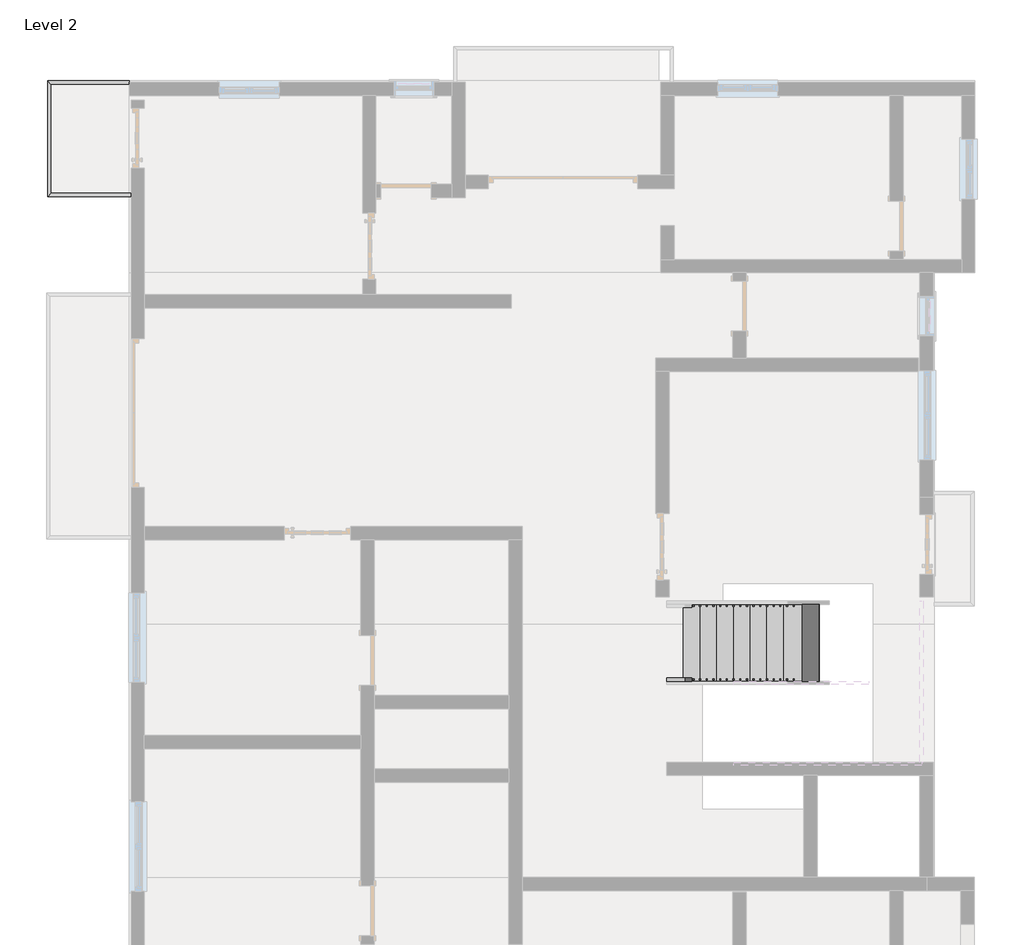
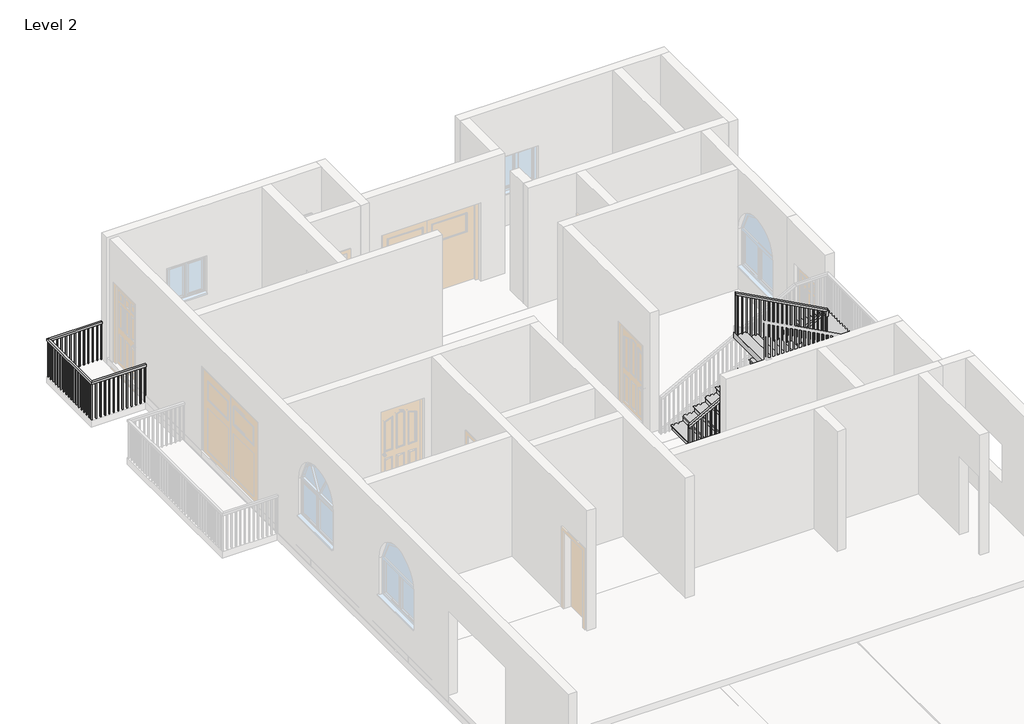
# One storey, part 5 of 7: 2 railings, 1 stair flight.
"""IFC4 building model written with IfcOpenShell, lengths in millimetres."""

from ifc_helpers import new_model, si_unit, frame, origin, place, context, project, spatial, polyline, outline, extrude, faceted_brep, transform, mapped, element, save
from components import stair_flight_e3e94c6b

model = new_model("IFC4")

# Units and contexts
model_context = context("Model", 3, world=origin())
ifc_project = project(units=[si_unit("LENGTHUNIT", "METRE", prefix="MILLI")], contexts=[model_context])

# Site, building, storey
site = spatial("IfcSite", under=ifc_project)
building = spatial("IfcBuilding", under=site)
storey = spatial("IfcBuildingStorey", under=building, Name="Level 2", Elevation=3048.0)

# Railings
placement = place(None, origin())
element("IfcRailing", 1, ObjectType="Handrail - Rectangular", at=placement, inside=storey, context=model_context, shape_type="SolidModel", body=[
    faceted_brep([(-6354.2109037, 9376.4527313, 3962.4), (-6354.2109037, 9376.4527313, 3911.6), (-6354.2109037, 9427.2527313, 3911.6), (-6354.2109037, 9427.2527313, 3962.4), (-7548.0109037, 9376.4527313, 3962.4), (-7548.0109037, 9376.4527313, 3911.6), (-7598.8109037, 9427.2527313, 3911.6), (-7598.8109037, 9427.2527313, 3962.4), (-7548.0109037, 7717.9584215, 3962.4), (-7548.0109037, 7717.9584215, 3911.6), (-7598.8109037, 7667.1584215, 3911.6), (-7598.8109037, 7667.1584215, 3962.4), (-6330.8013636, 7717.9584215, 3962.4), (-6330.8013636, 7667.1584215, 3962.4), (-6330.8013636, 7667.1584215, 3911.6), (-6330.8013636, 7717.9584215, 3911.6)], [[[0, 1, 2, 3]], [[1, 0, 4, 5]], [[2, 1, 5, 6]], [[3, 2, 6, 7]], [[0, 3, 7, 4]], [[5, 4, 8, 9]], [[6, 5, 9, 10]], [[7, 6, 10, 11]], [[4, 7, 11, 8]], [[12, 13, 14, 15]], [[9, 8, 12, 15]], [[10, 9, 15, 14]], [[11, 10, 14, 13]], [[8, 11, 13, 12]]]),
    extrude(outline(polyline([(-6363.7359037, 7683.0334215), (-6363.7359037, 7702.0834215), (-6344.6859037, 7702.0834215), (-6344.6859037, 7683.0334215), (-6363.7359037, 7683.0334215)])), frame((0.0, 0.0, 3048.0), z_axis=(0.0, 0.0, 1.0), x_axis=(1.0, 0.0, 0.0)), (0.0, 0.0, 1.0), 863.6),
    extrude(outline(polyline([(-6465.3359037, 7683.0334215), (-6465.3359037, 7702.0834215), (-6446.2859037, 7702.0834215), (-6446.2859037, 7683.0334215), (-6465.3359037, 7683.0334215)])), frame((0.0, 0.0, 3048.0), z_axis=(0.0, 0.0, 1.0), x_axis=(1.0, 0.0, 0.0)), (0.0, 0.0, 1.0), 863.6),
    extrude(outline(polyline([(-6566.9359037, 7683.0334215), (-6566.9359037, 7702.0834215), (-6547.8859037, 7702.0834215), (-6547.8859037, 7683.0334215), (-6566.9359037, 7683.0334215)])), frame((0.0, 0.0, 3048.0), z_axis=(0.0, 0.0, 1.0), x_axis=(1.0, 0.0, 0.0)), (0.0, 0.0, 1.0), 863.6),
    extrude(outline(polyline([(-6668.5359037, 7683.0334215), (-6668.5359037, 7702.0834215), (-6649.4859037, 7702.0834215), (-6649.4859037, 7683.0334215), (-6668.5359037, 7683.0334215)])), frame((0.0, 0.0, 3048.0), z_axis=(0.0, 0.0, 1.0), x_axis=(1.0, 0.0, 0.0)), (0.0, 0.0, 1.0), 863.6),
    extrude(outline(polyline([(-6770.1359037, 7683.0334215), (-6770.1359037, 7702.0834215), (-6751.0859037, 7702.0834215), (-6751.0859037, 7683.0334215), (-6770.1359037, 7683.0334215)])), frame((0.0, 0.0, 3048.0), z_axis=(0.0, 0.0, 1.0), x_axis=(1.0, 0.0, 0.0)), (0.0, 0.0, 1.0), 863.6),
    extrude(outline(polyline([(-6871.7359037, 7683.0334215), (-6871.7359037, 7702.0834215), (-6852.6859037, 7702.0834215), (-6852.6859037, 7683.0334215), (-6871.7359037, 7683.0334215)])), frame((0.0, 0.0, 3048.0), z_axis=(0.0, 0.0, 1.0), x_axis=(1.0, 0.0, 0.0)), (0.0, 0.0, 1.0), 863.6),
    extrude(outline(polyline([(-6973.3359037, 7683.0334215), (-6973.3359037, 7702.0834215), (-6954.2859037, 7702.0834215), (-6954.2859037, 7683.0334215), (-6973.3359037, 7683.0334215)])), frame((0.0, 0.0, 3048.0), z_axis=(0.0, 0.0, 1.0), x_axis=(1.0, 0.0, 0.0)), (0.0, 0.0, 1.0), 863.6),
    extrude(outline(polyline([(-7074.9359037, 7683.0334215), (-7074.9359037, 7702.0834215), (-7055.8859037, 7702.0834215), (-7055.8859037, 7683.0334215), (-7074.9359037, 7683.0334215)])), frame((0.0, 0.0, 3048.0), z_axis=(0.0, 0.0, 1.0), x_axis=(1.0, 0.0, 0.0)), (0.0, 0.0, 1.0), 863.6),
    extrude(outline(polyline([(-7176.5359037, 7683.0334215), (-7176.5359037, 7702.0834215), (-7157.4859037, 7702.0834215), (-7157.4859037, 7683.0334215), (-7176.5359037, 7683.0334215)])), frame((0.0, 0.0, 3048.0), z_axis=(0.0, 0.0, 1.0), x_axis=(1.0, 0.0, 0.0)), (0.0, 0.0, 1.0), 863.6),
    extrude(outline(polyline([(-7278.1359037, 7683.0334215), (-7278.1359037, 7702.0834215), (-7259.0859037, 7702.0834215), (-7259.0859037, 7683.0334215), (-7278.1359037, 7683.0334215)])), frame((0.0, 0.0, 3048.0), z_axis=(0.0, 0.0, 1.0), x_axis=(1.0, 0.0, 0.0)), (0.0, 0.0, 1.0), 863.6),
    extrude(outline(polyline([(-7379.7359037, 7683.0334215), (-7379.7359037, 7702.0834215), (-7360.6859037, 7702.0834215), (-7360.6859037, 7683.0334215), (-7379.7359037, 7683.0334215)])), frame((0.0, 0.0, 3048.0), z_axis=(0.0, 0.0, 1.0), x_axis=(1.0, 0.0, 0.0)), (0.0, 0.0, 1.0), 863.6),
    extrude(outline(polyline([(-7481.3359037, 7683.0334215), (-7481.3359037, 7702.0834215), (-7462.2859037, 7702.0834215), (-7462.2859037, 7683.0334215), (-7481.3359037, 7683.0334215)])), frame((0.0, 0.0, 3048.0), z_axis=(0.0, 0.0, 1.0), x_axis=(1.0, 0.0, 0.0)), (0.0, 0.0, 1.0), 863.6),
    extrude(outline(polyline([(-7582.9359037, 7785.7777313), (-7563.8859037, 7785.7777313), (-7563.8859037, 7766.7277313), (-7582.9359037, 7766.7277313), (-7582.9359037, 7785.7777313)])), frame((0.0, 0.0, 3048.0), z_axis=(0.0, 0.0, 1.0), x_axis=(1.0, 0.0, 0.0)), (0.0, 0.0, 1.0), 863.6),
    extrude(outline(polyline([(-7582.9359037, 7887.3777313), (-7563.8859037, 7887.3777313), (-7563.8859037, 7868.3277313), (-7582.9359037, 7868.3277313), (-7582.9359037, 7887.3777313)])), frame((0.0, 0.0, 3048.0), z_axis=(0.0, 0.0, 1.0), x_axis=(1.0, 0.0, 0.0)), (0.0, 0.0, 1.0), 863.6),
    extrude(outline(polyline([(-7582.9359037, 7988.9777313), (-7563.8859037, 7988.9777313), (-7563.8859037, 7969.9277313), (-7582.9359037, 7969.9277313), (-7582.9359037, 7988.9777313)])), frame((0.0, 0.0, 3048.0), z_axis=(0.0, 0.0, 1.0), x_axis=(1.0, 0.0, 0.0)), (0.0, 0.0, 1.0), 863.6),
    extrude(outline(polyline([(-7582.9359037, 8090.5777313), (-7563.8859037, 8090.5777313), (-7563.8859037, 8071.5277313), (-7582.9359037, 8071.5277313), (-7582.9359037, 8090.5777313)])), frame((0.0, 0.0, 3048.0), z_axis=(0.0, 0.0, 1.0), x_axis=(1.0, 0.0, 0.0)), (0.0, 0.0, 1.0), 863.6),
    extrude(outline(polyline([(-7582.9359037, 8192.1777313), (-7563.8859037, 8192.1777313), (-7563.8859037, 8173.1277313), (-7582.9359037, 8173.1277313), (-7582.9359037, 8192.1777313)])), frame((0.0, 0.0, 3048.0), z_axis=(0.0, 0.0, 1.0), x_axis=(1.0, 0.0, 0.0)), (0.0, 0.0, 1.0), 863.6),
    extrude(outline(polyline([(-7582.9359037, 8293.7777313), (-7563.8859037, 8293.7777313), (-7563.8859037, 8274.7277313), (-7582.9359037, 8274.7277313), (-7582.9359037, 8293.7777313)])), frame((0.0, 0.0, 3048.0), z_axis=(0.0, 0.0, 1.0), x_axis=(1.0, 0.0, 0.0)), (0.0, 0.0, 1.0), 863.6),
    extrude(outline(polyline([(-7582.9359037, 8395.3777313), (-7563.8859037, 8395.3777313), (-7563.8859037, 8376.3277313), (-7582.9359037, 8376.3277313), (-7582.9359037, 8395.3777313)])), frame((0.0, 0.0, 3048.0), z_axis=(0.0, 0.0, 1.0), x_axis=(1.0, 0.0, 0.0)), (0.0, 0.0, 1.0), 863.6),
    extrude(outline(polyline([(-7582.9359037, 8496.9777313), (-7563.8859037, 8496.9777313), (-7563.8859037, 8477.9277313), (-7582.9359037, 8477.9277313), (-7582.9359037, 8496.9777313)])), frame((0.0, 0.0, 3048.0), z_axis=(0.0, 0.0, 1.0), x_axis=(1.0, 0.0, 0.0)), (0.0, 0.0, 1.0), 863.6),
    extrude(outline(polyline([(-7582.9359037, 8598.5777313), (-7563.8859037, 8598.5777313), (-7563.8859037, 8579.5277313), (-7582.9359037, 8579.5277313), (-7582.9359037, 8598.5777313)])), frame((0.0, 0.0, 3048.0), z_axis=(0.0, 0.0, 1.0), x_axis=(1.0, 0.0, 0.0)), (0.0, 0.0, 1.0), 863.6),
    extrude(outline(polyline([(-7582.9359037, 8700.1777313), (-7563.8859037, 8700.1777313), (-7563.8859037, 8681.1277313), (-7582.9359037, 8681.1277313), (-7582.9359037, 8700.1777313)])), frame((0.0, 0.0, 3048.0), z_axis=(0.0, 0.0, 1.0), x_axis=(1.0, 0.0, 0.0)), (0.0, 0.0, 1.0), 863.6),
    extrude(outline(polyline([(-7582.9359037, 8801.7777313), (-7563.8859037, 8801.7777313), (-7563.8859037, 8782.7277313), (-7582.9359037, 8782.7277313), (-7582.9359037, 8801.7777313)])), frame((0.0, 0.0, 3048.0), z_axis=(0.0, 0.0, 1.0), x_axis=(1.0, 0.0, 0.0)), (0.0, 0.0, 1.0), 863.6),
    extrude(outline(polyline([(-7582.9359037, 8903.3777313), (-7563.8859037, 8903.3777313), (-7563.8859037, 8884.3277313), (-7582.9359037, 8884.3277313), (-7582.9359037, 8903.3777313)])), frame((0.0, 0.0, 3048.0), z_axis=(0.0, 0.0, 1.0), x_axis=(1.0, 0.0, 0.0)), (0.0, 0.0, 1.0), 863.6),
    extrude(outline(polyline([(-7582.9359037, 9004.9777313), (-7563.8859037, 9004.9777313), (-7563.8859037, 8985.9277313), (-7582.9359037, 8985.9277313), (-7582.9359037, 9004.9777313)])), frame((0.0, 0.0, 3048.0), z_axis=(0.0, 0.0, 1.0), x_axis=(1.0, 0.0, 0.0)), (0.0, 0.0, 1.0), 863.6),
    extrude(outline(polyline([(-7582.9359037, 9106.5777313), (-7563.8859037, 9106.5777313), (-7563.8859037, 9087.5277313), (-7582.9359037, 9087.5277313), (-7582.9359037, 9106.5777313)])), frame((0.0, 0.0, 3048.0), z_axis=(0.0, 0.0, 1.0), x_axis=(1.0, 0.0, 0.0)), (0.0, 0.0, 1.0), 863.6),
    extrude(outline(polyline([(-7582.9359037, 9208.1777313), (-7563.8859037, 9208.1777313), (-7563.8859037, 9189.1277313), (-7582.9359037, 9189.1277313), (-7582.9359037, 9208.1777313)])), frame((0.0, 0.0, 3048.0), z_axis=(0.0, 0.0, 1.0), x_axis=(1.0, 0.0, 0.0)), (0.0, 0.0, 1.0), 863.6),
    extrude(outline(polyline([(-7582.9359037, 9309.7777313), (-7563.8859037, 9309.7777313), (-7563.8859037, 9290.7277313), (-7582.9359037, 9290.7277313), (-7582.9359037, 9309.7777313)])), frame((0.0, 0.0, 3048.0), z_axis=(0.0, 0.0, 1.0), x_axis=(1.0, 0.0, 0.0)), (0.0, 0.0, 1.0), 863.6),
    extrude(outline(polyline([(-7462.2859037, 9411.3777313), (-7462.2859037, 9392.3277313), (-7481.3359037, 9392.3277313), (-7481.3359037, 9411.3777313), (-7462.2859037, 9411.3777313)])), frame((0.0, 0.0, 3048.0), z_axis=(0.0, 0.0, 1.0), x_axis=(1.0, 0.0, 0.0)), (0.0, 0.0, 1.0), 863.6),
    extrude(outline(polyline([(-7360.6859037, 9411.3777313), (-7360.6859037, 9392.3277313), (-7379.7359037, 9392.3277313), (-7379.7359037, 9411.3777313), (-7360.6859037, 9411.3777313)])), frame((0.0, 0.0, 3048.0), z_axis=(0.0, 0.0, 1.0), x_axis=(1.0, 0.0, 0.0)), (0.0, 0.0, 1.0), 863.6),
    extrude(outline(polyline([(-7259.0859037, 9411.3777313), (-7259.0859037, 9392.3277313), (-7278.1359037, 9392.3277313), (-7278.1359037, 9411.3777313), (-7259.0859037, 9411.3777313)])), frame((0.0, 0.0, 3048.0), z_axis=(0.0, 0.0, 1.0), x_axis=(1.0, 0.0, 0.0)), (0.0, 0.0, 1.0), 863.6),
    extrude(outline(polyline([(-7157.4859037, 9411.3777313), (-7157.4859037, 9392.3277313), (-7176.5359037, 9392.3277313), (-7176.5359037, 9411.3777313), (-7157.4859037, 9411.3777313)])), frame((0.0, 0.0, 3048.0), z_axis=(0.0, 0.0, 1.0), x_axis=(1.0, 0.0, 0.0)), (0.0, 0.0, 1.0), 863.6),
    extrude(outline(polyline([(-7055.8859037, 9411.3777313), (-7055.8859037, 9392.3277313), (-7074.9359037, 9392.3277313), (-7074.9359037, 9411.3777313), (-7055.8859037, 9411.3777313)])), frame((0.0, 0.0, 3048.0), z_axis=(0.0, 0.0, 1.0), x_axis=(1.0, 0.0, 0.0)), (0.0, 0.0, 1.0), 863.6),
    extrude(outline(polyline([(-6954.2859037, 9411.3777313), (-6954.2859037, 9392.3277313), (-6973.3359037, 9392.3277313), (-6973.3359037, 9411.3777313), (-6954.2859037, 9411.3777313)])), frame((0.0, 0.0, 3048.0), z_axis=(0.0, 0.0, 1.0), x_axis=(1.0, 0.0, 0.0)), (0.0, 0.0, 1.0), 863.6),
    extrude(outline(polyline([(-6852.6859037, 9411.3777313), (-6852.6859037, 9392.3277313), (-6871.7359037, 9392.3277313), (-6871.7359037, 9411.3777313), (-6852.6859037, 9411.3777313)])), frame((0.0, 0.0, 3048.0), z_axis=(0.0, 0.0, 1.0), x_axis=(1.0, 0.0, 0.0)), (0.0, 0.0, 1.0), 863.6),
    extrude(outline(polyline([(-6751.0859037, 9411.3777313), (-6751.0859037, 9392.3277313), (-6770.1359037, 9392.3277313), (-6770.1359037, 9411.3777313), (-6751.0859037, 9411.3777313)])), frame((0.0, 0.0, 3048.0), z_axis=(0.0, 0.0, 1.0), x_axis=(1.0, 0.0, 0.0)), (0.0, 0.0, 1.0), 863.6),
    extrude(outline(polyline([(-6649.4859037, 9411.3777313), (-6649.4859037, 9392.3277313), (-6668.5359037, 9392.3277313), (-6668.5359037, 9411.3777313), (-6649.4859037, 9411.3777313)])), frame((0.0, 0.0, 3048.0), z_axis=(0.0, 0.0, 1.0), x_axis=(1.0, 0.0, 0.0)), (0.0, 0.0, 1.0), 863.6),
    extrude(outline(polyline([(-6547.8859037, 9411.3777313), (-6547.8859037, 9392.3277313), (-6566.9359037, 9392.3277313), (-6566.9359037, 9411.3777313), (-6547.8859037, 9411.3777313)])), frame((0.0, 0.0, 3048.0), z_axis=(0.0, 0.0, 1.0), x_axis=(1.0, 0.0, 0.0)), (0.0, 0.0, 1.0), 863.6),
    extrude(outline(polyline([(-6446.2859037, 9411.3777313), (-6446.2859037, 9392.3277313), (-6465.3359037, 9392.3277313), (-6465.3359037, 9411.3777313), (-6446.2859037, 9411.3777313)])), frame((0.0, 0.0, 3048.0), z_axis=(0.0, 0.0, 1.0), x_axis=(1.0, 0.0, 0.0)), (0.0, 0.0, 1.0), 863.6),
    extrude(outline(polyline([(-7582.9359037, 7702.0834215), (-7563.8859037, 7702.0834215), (-7563.8859037, 7683.0334215), (-7582.9359037, 7683.0334215), (-7582.9359037, 7702.0834215)])), frame((0.0, 0.0, 3048.0), z_axis=(0.0, 0.0, 1.0), x_axis=(1.0, 0.0, 0.0)), (0.0, 0.0, 1.0), 863.6),
    extrude(outline(polyline([(-7563.8859037, 9411.3777313), (-7563.8859037, 9392.3277313), (-7582.9359037, 9392.3277313), (-7582.9359037, 9411.3777313), (-7563.8859037, 9411.3777313)])), frame((0.0, 0.0, 3048.0), z_axis=(0.0, 0.0, 1.0), x_axis=(1.0, 0.0, 0.0)), (0.0, 0.0, 1.0), 863.6),
    extrude(outline(polyline([(-6349.8513636, 7683.0334215), (-6349.8513636, 7702.0834215), (-6330.8013636, 7702.0834215), (-6330.8013636, 7683.0334215), (-6349.8513636, 7683.0334215)])), frame((0.0, 0.0, 3048.0), z_axis=(0.0, 0.0, 1.0), x_axis=(1.0, 0.0, 0.0)), (0.0, 0.0, 1.0), 863.6),
    extrude(outline(polyline([(-6354.2109037, 9411.3777313), (-6354.2109037, 9392.3277313), (-6373.2609037, 9392.3277313), (-6373.2609037, 9411.3777313), (-6354.2109037, 9411.3777313)])), frame((0.0, 0.0, 3048.0), z_axis=(0.0, 0.0, 1.0), x_axis=(1.0, 0.0, 0.0)), (0.0, 0.0, 1.0), 863.6),
])
element("IfcRailing", 2, ObjectType="Handrail - Rectangular", at=placement, inside=storey, context=model_context, shape_type="SolidModel", body=[
    faceted_brep([(1811.8890963, 347.1962251, 4100.9454545), (1811.8890963, 347.1962251, 4043.1709673), (1811.8890963, 296.3962251, 4043.1709673), (1811.8890963, 296.3962251, 4100.9454545), (4804.8326586, 347.1962251, 5722.2136078), (4855.6326586, 347.1962251, 5691.9573214), (4855.6326586, 296.3962251, 5691.9573214), (4804.8326586, 296.3962251, 5722.2136078), (4804.8326586, 347.1962251, 5763.4909091), (4855.6326586, 347.1962251, 5712.6909091), (4855.6326586, 296.3962251, 5712.6909091), (4804.8326586, 296.3962251, 5763.4909091), (4931.8326586, 347.1962251, 5763.4909091), (4931.8326586, 347.1962251, 5712.6909091), (4881.0326586, 296.3962251, 5712.6909091), (4881.0326586, 296.3962251, 5763.4909091), (4931.8326586, 245.5962251, 5763.4909091), (4881.0326586, 245.5962251, 5763.4909091), (4881.0326586, 194.7962251, 5712.6909091), (4931.8326586, 194.7962251, 5712.6909091)], [[[0, 1, 2, 3]], [[1, 0, 4, 5]], [[2, 1, 5, 6]], [[3, 2, 6, 7]], [[0, 3, 7, 4]], [[5, 4, 8, 9]], [[6, 5, 9, 10]], [[7, 6, 10, 11]], [[4, 7, 11, 8]], [[9, 8, 12, 13]], [[10, 9, 13, 14]], [[11, 10, 14, 15]], [[8, 11, 15, 12]], [[16, 17, 18, 19]], [[13, 12, 16, 19]], [[14, 13, 19, 18]], [[15, 14, 18, 17]], [[12, 15, 17, 16]]]),
    faceted_brep([(4931.8326586, 245.5962251, 5763.4909091), (4931.8326586, 194.7962251, 5712.6909091), (4881.0326586, 194.7962251, 5712.6909091), (4881.0326586, 245.5962251, 5763.4909091), (4931.8326586, 245.5962251, 5874.6126249), (4881.0326586, 245.5962251, 5844.3068093), (4881.0326586, 194.7962251, 5844.3068093), (4931.8326586, 194.7962251, 5874.6126249)], [[[0, 1, 2, 3]], [[4, 5, 6, 7]], [[1, 0, 4, 7]], [[2, 1, 7, 6]], [[3, 2, 6, 5]], [[0, 3, 5, 4]]]),
    faceted_brep([(4931.8326586, 194.7962251, 5874.6126249), (4881.0326586, 194.7962251, 5844.3068093), (4881.0326586, 245.5962251, 5844.3068093), (4931.8326586, 245.5962251, 5874.6126249), (2827.8890963, 194.7962251, 7010.4), (2827.8890963, 245.5962251, 7010.4), (2827.8890963, 245.5962251, 6952.6704456), (2827.8890963, 194.7962251, 6952.6704456)], [[[0, 1, 2, 3]], [[4, 5, 6, 7]], [[1, 0, 4, 7]], [[2, 1, 7, 6]], [[3, 2, 6, 5]], [[0, 3, 5, 4]]]),
    extrude(outline(polyline([(6922.40254, 2883.9576586), (6932.686442, 2864.9076586), (5957.4545455, 2864.9076586), (5957.4545455, 2883.9576586), (6922.40254, 2883.9576586)])), frame((0.0, 210.6712251, 0.0), z_axis=(0.0, 1.0, 0.0), x_axis=(0.0, 0.0, 1.0)), (0.0, 0.0, 1.0), 19.05),
    extrude(outline(polyline([(6867.5550624, 2985.5576586), (6877.8389645, 2966.5076586), (5957.4545455, 2966.5076586), (5957.4545455, 2985.5576586), (6867.5550624, 2985.5576586)])), frame((0.0, 210.6712251, 0.0), z_axis=(0.0, 1.0, 0.0), x_axis=(0.0, 0.0, 1.0)), (0.0, 0.0, 1.0), 19.05),
    extrude(outline(polyline([(6812.7075849, 3087.1576586), (6822.9914869, 3068.1076586), (5957.4545455, 3068.1076586), (5957.4545455, 3087.1576586), (6812.7075849, 3087.1576586)])), frame((0.0, 210.6712251, 0.0), z_axis=(0.0, 1.0, 0.0), x_axis=(0.0, 0.0, 1.0)), (0.0, 0.0, 1.0), 19.05),
    extrude(outline(polyline([(6757.8601073, 3188.7576586), (6768.1440094, 3169.7076586), (5818.9090909, 3169.7076586), (5818.9090909, 3188.7576586), (6757.8601073, 3188.7576586)])), frame((0.0, 210.6712251, 0.0), z_axis=(0.0, 1.0, 0.0), x_axis=(0.0, 0.0, 1.0)), (0.0, 0.0, 1.0), 19.05),
    extrude(outline(polyline([(6703.0126298, 3290.3576586), (6713.2965318, 3271.3076586), (5818.9090909, 3271.3076586), (5818.9090909, 3290.3576586), (6703.0126298, 3290.3576586)])), frame((0.0, 210.6712251, 0.0), z_axis=(0.0, 1.0, 0.0), x_axis=(0.0, 0.0, 1.0)), (0.0, 0.0, 1.0), 19.05),
    extrude(outline(polyline([(6648.1651522, 3391.9576586), (6658.4490542, 3372.9076586), (5680.3636364, 3372.9076586), (5680.3636364, 3391.9576586), (6648.1651522, 3391.9576586)])), frame((0.0, 210.6712251, 0.0), z_axis=(0.0, 1.0, 0.0), x_axis=(0.0, 0.0, 1.0)), (0.0, 0.0, 1.0), 19.05),
    extrude(outline(polyline([(6593.3176746, 3493.5576586), (6603.6015767, 3474.5076586), (5680.3636364, 3474.5076586), (5680.3636364, 3493.5576586), (6593.3176746, 3493.5576586)])), frame((0.0, 210.6712251, 0.0), z_axis=(0.0, 1.0, 0.0), x_axis=(0.0, 0.0, 1.0)), (0.0, 0.0, 1.0), 19.05),
    extrude(outline(polyline([(6538.4701971, 3595.1576586), (6548.7540991, 3576.1076586), (5680.3636364, 3576.1076586), (5680.3636364, 3595.1576586), (6538.4701971, 3595.1576586)])), frame((0.0, 210.6712251, 0.0), z_axis=(0.0, 1.0, 0.0), x_axis=(0.0, 0.0, 1.0)), (0.0, 0.0, 1.0), 19.05),
    extrude(outline(polyline([(6483.6227195, 3696.7576586), (6493.9066216, 3677.7076586), (5541.8181818, 3677.7076586), (5541.8181818, 3696.7576586), (6483.6227195, 3696.7576586)])), frame((0.0, 210.6712251, 0.0), z_axis=(0.0, 1.0, 0.0), x_axis=(0.0, 0.0, 1.0)), (0.0, 0.0, 1.0), 19.05),
    extrude(outline(polyline([(6428.775242, 3798.3576586), (6439.059144, 3779.3076586), (5541.8181818, 3779.3076586), (5541.8181818, 3798.3576586), (6428.775242, 3798.3576586)])), frame((0.0, 210.6712251, 0.0), z_axis=(0.0, 1.0, 0.0), x_axis=(0.0, 0.0, 1.0)), (0.0, 0.0, 1.0), 19.05),
    extrude(outline(polyline([(6373.9277644, 3899.9576586), (6384.2116665, 3880.9076586), (5403.2727273, 3880.9076586), (5403.2727273, 3899.9576586), (6373.9277644, 3899.9576586)])), frame((0.0, 210.6712251, 0.0), z_axis=(0.0, 1.0, 0.0), x_axis=(0.0, 0.0, 1.0)), (0.0, 0.0, 1.0), 19.05),
    extrude(outline(polyline([(6319.0802869, 4001.5576586), (6329.3641889, 3982.5076586), (5403.2727273, 3982.5076586), (5403.2727273, 4001.5576586), (6319.0802869, 4001.5576586)])), frame((0.0, 210.6712251, 0.0), z_axis=(0.0, 1.0, 0.0), x_axis=(0.0, 0.0, 1.0)), (0.0, 0.0, 1.0), 19.05),
    extrude(outline(polyline([(6264.2328093, 4103.1576586), (6274.5167113, 4084.1076586), (5403.2727273, 4084.1076586), (5403.2727273, 4103.1576586), (6264.2328093, 4103.1576586)])), frame((0.0, 210.6712251, 0.0), z_axis=(0.0, 1.0, 0.0), x_axis=(0.0, 0.0, 1.0)), (0.0, 0.0, 1.0), 19.05),
    extrude(outline(polyline([(6209.3853317, 4204.7576586), (6219.6692338, 4185.7076586), (5264.7272727, 4185.7076586), (5264.7272727, 4204.7576586), (6209.3853317, 4204.7576586)])), frame((0.0, 210.6712251, 0.0), z_axis=(0.0, 1.0, 0.0), x_axis=(0.0, 0.0, 1.0)), (0.0, 0.0, 1.0), 19.05),
    extrude(outline(polyline([(6154.5378542, 4306.3576586), (6164.8217562, 4287.3076586), (5264.7272727, 4287.3076586), (5264.7272727, 4306.3576586), (6154.5378542, 4306.3576586)])), frame((0.0, 210.6712251, 0.0), z_axis=(0.0, 1.0, 0.0), x_axis=(0.0, 0.0, 1.0)), (0.0, 0.0, 1.0), 19.05),
    extrude(outline(polyline([(6099.6903766, 4407.9576586), (6109.9742787, 4388.9076586), (5126.1818182, 4388.9076586), (5126.1818182, 4407.9576586), (6099.6903766, 4407.9576586)])), frame((0.0, 210.6712251, 0.0), z_axis=(0.0, 1.0, 0.0), x_axis=(0.0, 0.0, 1.0)), (0.0, 0.0, 1.0), 19.05),
    extrude(outline(polyline([(6044.8428991, 4509.5576586), (6055.1268011, 4490.5076586), (5126.1818182, 4490.5076586), (5126.1818182, 4509.5576586), (6044.8428991, 4509.5576586)])), frame((0.0, 210.6712251, 0.0), z_axis=(0.0, 1.0, 0.0), x_axis=(0.0, 0.0, 1.0)), (0.0, 0.0, 1.0), 19.05),
    extrude(outline(polyline([(5989.9954215, 4611.1576586), (6000.2793236, 4592.1076586), (5126.1818182, 4592.1076586), (5126.1818182, 4611.1576586), (5989.9954215, 4611.1576586)])), frame((0.0, 210.6712251, 0.0), z_axis=(0.0, 1.0, 0.0), x_axis=(0.0, 0.0, 1.0)), (0.0, 0.0, 1.0), 19.05),
    extrude(outline(polyline([(5935.147944, 4712.7576586), (5945.431846, 4693.7076586), (4987.6363636, 4693.7076586), (4987.6363636, 4712.7576586), (5935.147944, 4712.7576586)])), frame((0.0, 210.6712251, 0.0), z_axis=(0.0, 1.0, 0.0), x_axis=(0.0, 0.0, 1.0)), (0.0, 0.0, 1.0), 19.05),
    extrude(outline(polyline([(5880.3004664, 4814.3576586), (5890.5843684, 4795.3076586), (4987.6363636, 4795.3076586), (4987.6363636, 4814.3576586), (5880.3004664, 4814.3576586)])), frame((0.0, 210.6712251, 0.0), z_axis=(0.0, 1.0, 0.0), x_axis=(0.0, 0.0, 1.0)), (0.0, 0.0, 1.0), 19.05),
    extrude(outline(polyline([(4850.3640963, 312.2712251), (4850.3640963, 331.3212251), (4869.4140963, 331.3212251), (4869.4140963, 312.2712251), (4850.3640963, 312.2712251)])), frame((0.0, 0.0, 4710.5454545), z_axis=(0.0, 0.0, 1.0), x_axis=(1.0, 0.0, 0.0)), (0.0, 0.0, 1.0), 1002.1454545),
    extrude(outline(polyline([(5644.3862812, 4767.8140963), (5634.0669559, 4748.7640963), (4710.5454545, 4748.7640963), (4710.5454545, 4767.8140963), (5644.3862812, 4767.8140963)])), frame((0.0, 312.2712251, 0.0), z_axis=(0.0, 1.0, 0.0), x_axis=(0.0, 0.0, 1.0)), (0.0, 0.0, 1.0), 19.05),
    extrude(outline(polyline([(5589.3498795, 4666.2140963), (5579.0305541, 4647.1640963), (4710.5454545, 4647.1640963), (4710.5454545, 4666.2140963), (5589.3498795, 4666.2140963)])), frame((0.0, 312.2712251, 0.0), z_axis=(0.0, 1.0, 0.0), x_axis=(0.0, 0.0, 1.0)), (0.0, 0.0, 1.0), 19.05),
    extrude(outline(polyline([(5534.3134777, 4564.6140963), (5523.9941524, 4545.5640963), (4572.0, 4545.5640963), (4572.0, 4564.6140963), (5534.3134777, 4564.6140963)])), frame((0.0, 312.2712251, 0.0), z_axis=(0.0, 1.0, 0.0), x_axis=(0.0, 0.0, 1.0)), (0.0, 0.0, 1.0), 19.05),
    extrude(outline(polyline([(5479.2770759, 4463.0140963), (5468.9577506, 4443.9640963), (4572.0, 4443.9640963), (4572.0, 4463.0140963), (5479.2770759, 4463.0140963)])), frame((0.0, 312.2712251, 0.0), z_axis=(0.0, 1.0, 0.0), x_axis=(0.0, 0.0, 1.0)), (0.0, 0.0, 1.0), 19.05),
    extrude(outline(polyline([(5424.2406742, 4361.4140963), (5413.9213488, 4342.3640963), (4572.0, 4342.3640963), (4572.0, 4361.4140963), (5424.2406742, 4361.4140963)])), frame((0.0, 312.2712251, 0.0), z_axis=(0.0, 1.0, 0.0), x_axis=(0.0, 0.0, 1.0)), (0.0, 0.0, 1.0), 19.05),
    extrude(outline(polyline([(5369.2042724, 4259.8140963), (5358.8849471, 4240.7640963), (4433.4545455, 4240.7640963), (4433.4545455, 4259.8140963), (5369.2042724, 4259.8140963)])), frame((0.0, 312.2712251, 0.0), z_axis=(0.0, 1.0, 0.0), x_axis=(0.0, 0.0, 1.0)), (0.0, 0.0, 1.0), 19.05),
    extrude(outline(polyline([(5314.1678706, 4158.2140963), (5303.8485453, 4139.1640963), (4433.4545455, 4139.1640963), (4433.4545455, 4158.2140963), (5314.1678706, 4158.2140963)])), frame((0.0, 312.2712251, 0.0), z_axis=(0.0, 1.0, 0.0), x_axis=(0.0, 0.0, 1.0)), (0.0, 0.0, 1.0), 19.05),
    extrude(outline(polyline([(5259.1314688, 4056.6140963), (5248.8121435, 4037.5640963), (4294.9090909, 4037.5640963), (4294.9090909, 4056.6140963), (5259.1314688, 4056.6140963)])), frame((0.0, 312.2712251, 0.0), z_axis=(0.0, 1.0, 0.0), x_axis=(0.0, 0.0, 1.0)), (0.0, 0.0, 1.0), 19.05),
    extrude(outline(polyline([(5204.0950671, 3955.0140963), (5193.7757417, 3935.9640963), (4294.9090909, 3935.9640963), (4294.9090909, 3955.0140963), (5204.0950671, 3955.0140963)])), frame((0.0, 312.2712251, 0.0), z_axis=(0.0, 1.0, 0.0), x_axis=(0.0, 0.0, 1.0)), (0.0, 0.0, 1.0), 19.05),
    extrude(outline(polyline([(5149.0586653, 3853.4140963), (5138.73934, 3834.3640963), (4294.9090909, 3834.3640963), (4294.9090909, 3853.4140963), (5149.0586653, 3853.4140963)])), frame((0.0, 312.2712251, 0.0), z_axis=(0.0, 1.0, 0.0), x_axis=(0.0, 0.0, 1.0)), (0.0, 0.0, 1.0), 19.05),
    extrude(outline(polyline([(5094.0222635, 3751.8140963), (5083.7029382, 3732.7640963), (4156.3636364, 3732.7640963), (4156.3636364, 3751.8140963), (5094.0222635, 3751.8140963)])), frame((0.0, 312.2712251, 0.0), z_axis=(0.0, 1.0, 0.0), x_axis=(0.0, 0.0, 1.0)), (0.0, 0.0, 1.0), 19.05),
    extrude(outline(polyline([(5038.9858618, 3650.2140963), (5028.6665364, 3631.1640963), (4156.3636364, 3631.1640963), (4156.3636364, 3650.2140963), (5038.9858618, 3650.2140963)])), frame((0.0, 312.2712251, 0.0), z_axis=(0.0, 1.0, 0.0), x_axis=(0.0, 0.0, 1.0)), (0.0, 0.0, 1.0), 19.05),
    extrude(outline(polyline([(4983.94946, 3548.6140963), (4973.6301347, 3529.5640963), (4017.8181818, 3529.5640963), (4017.8181818, 3548.6140963), (4983.94946, 3548.6140963)])), frame((0.0, 312.2712251, 0.0), z_axis=(0.0, 1.0, 0.0), x_axis=(0.0, 0.0, 1.0)), (0.0, 0.0, 1.0), 19.05),
    extrude(outline(polyline([(4928.9130582, 3447.0140963), (4918.5937329, 3427.9640963), (4017.8181818, 3427.9640963), (4017.8181818, 3447.0140963), (4928.9130582, 3447.0140963)])), frame((0.0, 312.2712251, 0.0), z_axis=(0.0, 1.0, 0.0), x_axis=(0.0, 0.0, 1.0)), (0.0, 0.0, 1.0), 19.05),
    extrude(outline(polyline([(4873.8766565, 3345.4140963), (4863.5573311, 3326.3640963), (4017.8181818, 3326.3640963), (4017.8181818, 3345.4140963), (4873.8766565, 3345.4140963)])), frame((0.0, 312.2712251, 0.0), z_axis=(0.0, 1.0, 0.0), x_axis=(0.0, 0.0, 1.0)), (0.0, 0.0, 1.0), 19.05),
    extrude(outline(polyline([(4818.8402547, 3243.8140963), (4808.5209294, 3224.7640963), (3879.2727273, 3224.7640963), (3879.2727273, 3243.8140963), (4818.8402547, 3243.8140963)])), frame((0.0, 312.2712251, 0.0), z_axis=(0.0, 1.0, 0.0), x_axis=(0.0, 0.0, 1.0)), (0.0, 0.0, 1.0), 19.05),
    extrude(outline(polyline([(4763.8038529, 3142.2140963), (4753.4845276, 3123.1640963), (3879.2727273, 3123.1640963), (3879.2727273, 3142.2140963), (4763.8038529, 3142.2140963)])), frame((0.0, 312.2712251, 0.0), z_axis=(0.0, 1.0, 0.0), x_axis=(0.0, 0.0, 1.0)), (0.0, 0.0, 1.0), 19.05),
    extrude(outline(polyline([(4708.7674512, 3040.6140963), (4698.4481258, 3021.5640963), (3740.7272727, 3021.5640963), (3740.7272727, 3040.6140963), (4708.7674512, 3040.6140963)])), frame((0.0, 312.2712251, 0.0), z_axis=(0.0, 1.0, 0.0), x_axis=(0.0, 0.0, 1.0)), (0.0, 0.0, 1.0), 19.05),
    extrude(outline(polyline([(4653.7310494, 2939.0140963), (4643.4117241, 2919.9640963), (3740.7272727, 2919.9640963), (3740.7272727, 2939.0140963), (4653.7310494, 2939.0140963)])), frame((0.0, 312.2712251, 0.0), z_axis=(0.0, 1.0, 0.0), x_axis=(0.0, 0.0, 1.0)), (0.0, 0.0, 1.0), 19.05),
    extrude(outline(polyline([(4598.6946476, 2837.4140963), (4588.3753223, 2818.3640963), (3740.7272727, 2818.3640963), (3740.7272727, 2837.4140963), (4598.6946476, 2837.4140963)])), frame((0.0, 312.2712251, 0.0), z_axis=(0.0, 1.0, 0.0), x_axis=(0.0, 0.0, 1.0)), (0.0, 0.0, 1.0), 19.05),
    extrude(outline(polyline([(4543.6582459, 2735.8140963), (4533.3389205, 2716.7640963), (3602.1818182, 2716.7640963), (3602.1818182, 2735.8140963), (4543.6582459, 2735.8140963)])), frame((0.0, 312.2712251, 0.0), z_axis=(0.0, 1.0, 0.0), x_axis=(0.0, 0.0, 1.0)), (0.0, 0.0, 1.0), 19.05),
    extrude(outline(polyline([(4488.6218441, 2634.2140963), (4478.3025188, 2615.1640963), (3602.1818182, 2615.1640963), (3602.1818182, 2634.2140963), (4488.6218441, 2634.2140963)])), frame((0.0, 312.2712251, 0.0), z_axis=(0.0, 1.0, 0.0), x_axis=(0.0, 0.0, 1.0)), (0.0, 0.0, 1.0), 19.05),
    extrude(outline(polyline([(4433.5854423, 2532.6140963), (4423.266117, 2513.5640963), (3463.6363636, 2513.5640963), (3463.6363636, 2532.6140963), (4433.5854423, 2532.6140963)])), frame((0.0, 312.2712251, 0.0), z_axis=(0.0, 1.0, 0.0), x_axis=(0.0, 0.0, 1.0)), (0.0, 0.0, 1.0), 19.05),
    extrude(outline(polyline([(4378.5490405, 2431.0140963), (4368.2297152, 2411.9640963), (3463.6363636, 2411.9640963), (3463.6363636, 2431.0140963), (4378.5490405, 2431.0140963)])), frame((0.0, 312.2712251, 0.0), z_axis=(0.0, 1.0, 0.0), x_axis=(0.0, 0.0, 1.0)), (0.0, 0.0, 1.0), 19.05),
    extrude(outline(polyline([(4323.5126388, 2329.4140963), (4313.1933134, 2310.3640963), (3463.6363636, 2310.3640963), (3463.6363636, 2329.4140963), (4323.5126388, 2329.4140963)])), frame((0.0, 312.2712251, 0.0), z_axis=(0.0, 1.0, 0.0), x_axis=(0.0, 0.0, 1.0)), (0.0, 0.0, 1.0), 19.05),
    extrude(outline(polyline([(4268.476237, 2227.8140963), (4258.1569117, 2208.7640963), (3325.0909091, 2208.7640963), (3325.0909091, 2227.8140963), (4268.476237, 2227.8140963)])), frame((0.0, 312.2712251, 0.0), z_axis=(0.0, 1.0, 0.0), x_axis=(0.0, 0.0, 1.0)), (0.0, 0.0, 1.0), 19.05),
    extrude(outline(polyline([(4213.4398352, 2126.2140963), (4203.1205099, 2107.1640963), (3325.0909091, 2107.1640963), (3325.0909091, 2126.2140963), (4213.4398352, 2126.2140963)])), frame((0.0, 312.2712251, 0.0), z_axis=(0.0, 1.0, 0.0), x_axis=(0.0, 0.0, 1.0)), (0.0, 0.0, 1.0), 19.05),
    extrude(outline(polyline([(4158.4034335, 2024.6140963), (4148.0841081, 2005.5640963), (3186.5454545, 2005.5640963), (3186.5454545, 2024.6140963), (4158.4034335, 2024.6140963)])), frame((0.0, 312.2712251, 0.0), z_axis=(0.0, 1.0, 0.0), x_axis=(0.0, 0.0, 1.0)), (0.0, 0.0, 1.0), 19.05),
    extrude(outline(polyline([(4103.3670317, 1923.0140963), (4093.0477064, 1903.9640963), (3186.5454545, 1903.9640963), (3186.5454545, 1923.0140963), (4103.3670317, 1923.0140963)])), frame((0.0, 312.2712251, 0.0), z_axis=(0.0, 1.0, 0.0), x_axis=(0.0, 0.0, 1.0)), (0.0, 0.0, 1.0), 19.05),
    extrude(outline(polyline([(4896.9076586, 229.7212251), (4915.9576586, 229.7212251), (4915.9576586, 210.6712251), (4896.9076586, 210.6712251), (4896.9076586, 229.7212251)])), frame((0.0, 0.0, 4849.0909091), z_axis=(0.0, 0.0, 1.0), x_axis=(1.0, 0.0, 0.0)), (0.0, 0.0, 1.0), 863.6),
    extrude(outline(polyline([(4896.9076586, 312.2712251), (4896.9076586, 331.3212251), (4915.9576586, 331.3212251), (4915.9576586, 312.2712251), (4896.9076586, 312.2712251)])), frame((0.0, 0.0, 4849.0909091), z_axis=(0.0, 0.0, 1.0), x_axis=(1.0, 0.0, 0.0)), (0.0, 0.0, 1.0), 863.6),
    extrude(outline(polyline([(6942.3865436, 2846.9390963), (6952.6704456, 2827.8890963), (5957.4545455, 2827.8890963), (5957.4545455, 2846.9390963), (6942.3865436, 2846.9390963)])), frame((0.0, 210.6712251, 0.0), z_axis=(0.0, 1.0, 0.0), x_axis=(0.0, 0.0, 1.0)), (0.0, 0.0, 1.0), 19.05),
    extrude(outline(polyline([(4053.4902926, 1830.9390963), (4043.1709673, 1811.8890963), (3186.5454545, 1811.8890963), (3186.5454545, 1830.9390963), (4053.4902926, 1830.9390963)])), frame((0.0, 312.2712251, 0.0), z_axis=(0.0, 1.0, 0.0), x_axis=(0.0, 0.0, 1.0)), (0.0, 0.0, 1.0), 19.05),
])

# Stair flight
stair_flight_shape = stair_flight_e3e94c6b(model_context)
element("IfcStairFlight", 3, ObjectType="2\" Tread 1\" Nosing 1/4\" Riser", at=placement, inside=storey, context=model_context, shape_type="MappedRepresentation", body=[
    mapped(stair_flight_shape, transform((0.0, 0.0, 0.0), x_axis=(1.0, 0.0, 0.0), y_axis=(0.0, 1.0, 0.0), z_axis=(0.0, 0.0, 1.0))),
])

save(model, "model.ifc")

# Revit data of these elements
# Type "Handrail - Rectangular"
#   Assembly Code = "C2010400"
#   built-in parameter 1008612 = 0.0416667 (stored number, unit not read)
#   built-in parameter 1008611 = 0.0416667 (stored number, unit not read)
#   built-in parameter 1008609 = 0.333333 (stored number, unit not read)
#   built-in parameter 1008604 = 0.166667 (stored number, unit not read)
#   built-in parameter 1008603 = 0.166667 (stored number, unit not read)
#   Railing Height = 3' - 0"
#   built-in parameter 1008630 = 2
#   built-in parameter 1008610 = 2
#   built-in parameter 1008618 = Baluster - Square : 3/4"
# Elements 1, 2 (IfcRailing, "Handrail - Rectangular")
#   Phase Created = New Construction
# Element 3 (IfcStairFlight, "2\" Tread 1\" Nosing 1/4\" Riser")
#   Phase Created = New Construction
